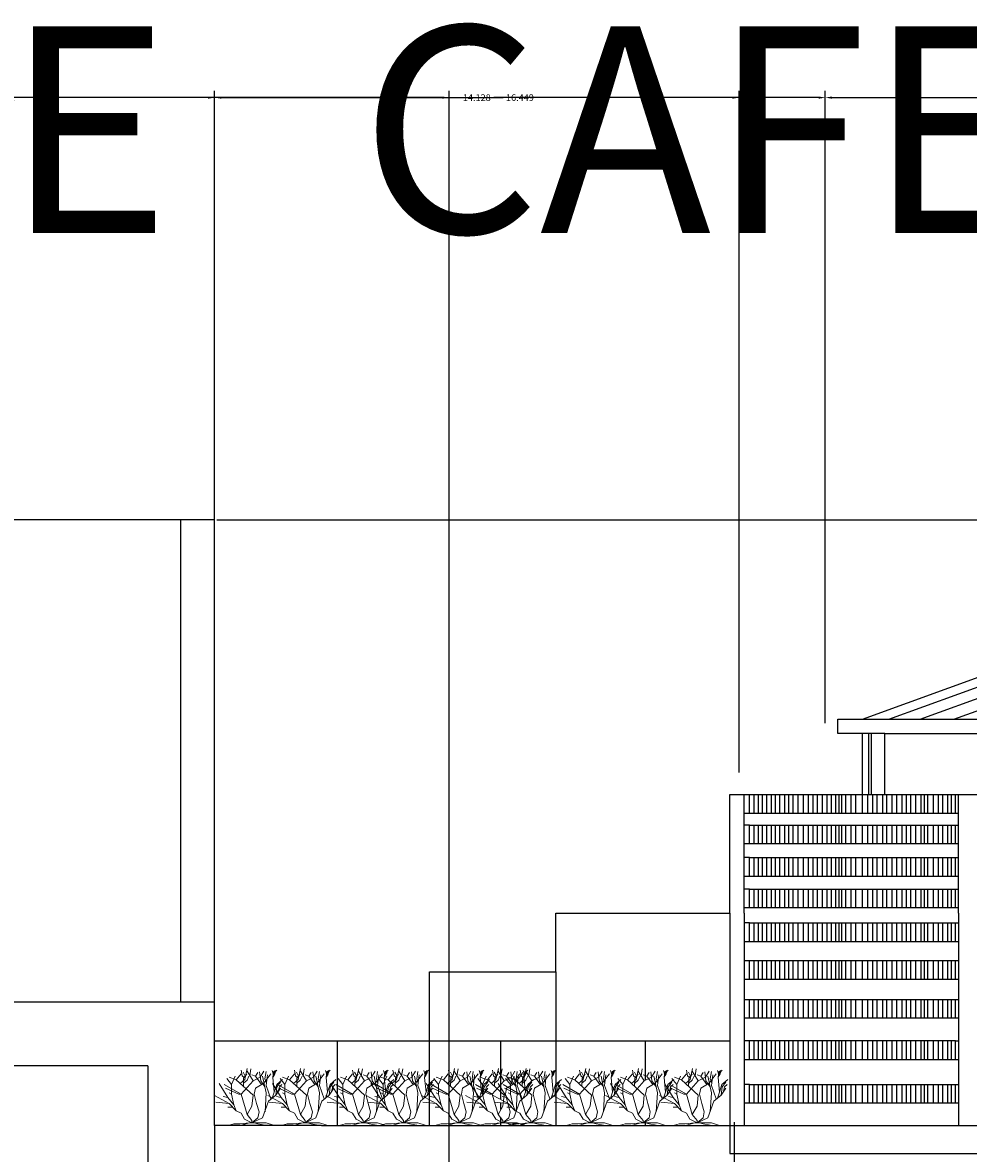
# Model space of a CAD drawing. Units: inches. Extents: x -117 to 121, y -77 to 40.
# Tile 30 of 45: x 9 to 34, y 10 to 40. Entities that reach past the tile are written whole.
import ezdxf

# ---------------------------------------------------------------- set-up
doc = ezdxf.new("R2010")
doc.units = ezdxf.units.IN
doc.header["$MEASUREMENT"] = 0
for name, color, linetype, lineweight in [('A-ANNO-DIMS', 2, 'Continuous', 18), ('A-ANNO-TEXT', 7, 'Continuous', 25), ('A-ELEV', 7, 'Continuous', 25), ('L-PLNT', 3, 'Continuous', 13)]:
    doc.layers.add(name, color=color, linetype=linetype, lineweight=lineweight)
doc.styles.get("Standard").update_dxf_attribs({"font": 'arial.ttf'})
doc.dimstyles.get("Standard").update_dxf_attribs({"dimtxt": 0.18, "dimasz": 0.18, "dimexe": 0.18, "dimexo": 0.0625, "dimgap": 0.09, "dimtad": 0, "dimtih": 1, "dimtoh": 1, "dimdec": 4, "dimzin": 0, "dimdsep": 46, "dimtxsty": 'Standard', "dimcen": 0.09, "dimadec": 0, "dimazin": 0, "dimtfac": 1, "dimtdec": 4, "dimtofl": 0, "dimtmove": 0, "dimatfit": 3, "dimfxl": 1, "dimtolj": 1, "dimtzin": 0, "dimarcsym": 0})

# ---------------------------------------------------------------- blocks, each defined once
blk = doc.blocks.new('*U3')
for p, q in [((-11.433, 18.289), (-10.457, 22.749)), ((-16.8, 16.32), (-18.72, 18.72)), ((-14.88, 18.24), (-17.76, 19.2)), ((-16.8, 16.32), (-15.36, 19.68)), ((-14.88, 18.24), (-12.96, 20.64)), ((-8.16, 12), (-14.88, 18.24)), ((-13.325, 16.724), (-11.433, 18.289)), ((-12.471, 19.775), (-12.898, 22.044)), ((-11.677, 19.071), (-12.471, 19.775)), ((-11.28, 19.619), (-12.104, 21.184)), ((-12.043, 15.628), (-11.921, 18.836)), ((-11.921, 18.836), (-10.64, 20.401)), ((-10.579, 18.054), (-9.846, 19.697)), ((-8.16, 17.76), (-10.56, 21.6)), ((-9.48, 19.775), (-8.992, 22.592)), ((-7.2, 19.68), (-8.64, 20.16)), ((-8.16, 17.76), (-5.28, 19.2)), ((-7.2, 19.68), (-6.24, 21.12)), ((-4.8, 16.32), (-7.2, 19.68)), ((-5.086, 17.741), (-5.513, 21.34)), ((-5.28, 19.2), (-3.84, 21.6)), ((-2.88, 12.96), (-4.32, 19.68)), ((-3.84, 16.8), (-0.96, 20.64)), ((-3.377, 18.602), (-2.888, 21.575)), ((-2.766, 16.802), (-3.377, 18.602)), ((-2.88, 15.84), (-2.4, 20.16)), ((-0.508, 21.888), (-0.081, 20.558)), ((-0.203, 19.149), (0.102, 21.34)), ((0.346, 13.203), (-0.203, 19.149)), ((-0.142, 19.384), (0.59, 20.401)), ((-0.02, 20.01), (0.896, 21.105)), ((0.041, 20.714), (1.384, 22.044)), ((0.102, 21.34), (0.835, 21.888)), ((1.323, 16.254), (3.642, 18.289)), ((-18.24, 11.04), (-21.755, 16.655)), ((-12.96, 12.48), (-19.68, 16.32)), ((-13.92, 12.48), (-19.2, 14.88)), ((-16.8, 12.48), (-16.8, 16.32)), ((-12.96, 12.48), (-8.16, 17.76)), ((-11.982, 16.802), (-10.579, 18.054)), ((-7.68, 12.48), (-7.2, 14.88)), ((-7.2, 14.88), (-3.84, 16.8)), ((-3.377, 15.315), (-5.086, 17.819)), ((-0.96, 10.56), (-2.88, 15.84)), ((0.346, 13.203), (1.323, 16.254)), ((0.96, 12), (1.44, 15.36)), ((0.96, 12), (2.88, 14.88)), ((1.44, 15.36), (2.88, 17.28)), ((1.92, 13.44), (2.4, 15.36)), ((2.4, 15.36), (3.36, 16.32)), ((-17.76, 8.64), (-23.663, 11.961)), ((-17.76, 8.64), (-23.128, 9.222)), ((-18.24, 11.04), (-20.16, 11.52)), ((-15.84, 8.16), (-18.24, 11.04)), ((-16.8, 12.48), (-17.76, 12.96)), ((-15.84, 8.16), (-16.8, 12.48)), ((-12.96, 12.48), (-13.92, 12.48)), ((-10.56, 4.32), (-12.96, 12.48)), ((-8.64, 7.68), (-8.16, 12)), ((-6.72, 8.64), (-7.68, 12.48)), ((-4.32, 2.88), (-1.92, 9.6)), ((-3.36, 5.28), (-2.88, 12.96)), ((-1.92, 9.6), (0.96, 12)), ((-0.48, 10.8), (0.346, 13.203)), ((-16.32, 7.2), (-18.24, 7.2)), ((-14.88, 5.76), (-17.76, 8.64)), ((-14.88, 5.76), (-15.84, 8.16)), ((-12.96, 4.8), (-14.88, 5.76)), ((-11.52, 2.4), (-12.96, 4.8)), ((-10.56, 4.32), (-8.64, 7.68)), ((-5.76, 5.28), (-6.72, 8.64)), ((-6.24, 2.88), (-5.76, 5.28)), ((-15.84, 0.48), (-17.76, 0)), ((-13.44, 0.48), (-15.84, 0.48)), ((-9.6, 0.96), (-13.44, 0.48)), ((-9.6, 0.96), (-12.96, 0)), ((-8.64, 0.96), (-11.52, 2.4)), ((-8.64, 1.92), (-10.56, 4.32)), ((-9.6, 0.96), (-7.68, 0.96)), ((-8.64, 0.96), (-4.32, 2.88)), ((-8.64, 0.96), (-6.24, 2.88)), ((-8.64, 0.96), (-8.64, 1.92)), ((-8.64, 0.96), (-2.88, 0.96)), ((-7.68, 0.96), (-6.24, 0.48)), ((-6.24, 0.48), (-3.36, 0)), ((-2.88, 0.96), (0, 0))]:
    blk.add_line(p, q)
blk = doc.blocks.new('*D10')
at = {"layer": 'A-ANNO-DIMS', "color": 0, "lineweight": -2, "transparency": 16777216}
for p, q in [((-2.6, 27.126), (-2.6, 38.61)), ((-2.42, 38.43), (5.304, 38.43)), ((13.798, 38.43), (6.075, 38.43)), ((13.978, 27.126), (13.978, 38.61))]:
    blk.add_line(p, q, dxfattribs=at)
at = {"layer": 'A-ANNO-DIMS', "color": 0, "transparency": 16777216}
for points in [[(-2.42, 38.46), (-2.42, 38.4), (-2.6, 38.43)], [(13.798, 38.46), (13.798, 38.4), (13.978, 38.43)]]:
    blk.add_solid(points, dxfattribs=at)
at = {"layer": 'Defpoints', "color": 0, "transparency": 16777216}
for p in [(13.978, 38.43), (-2.6, 27.063), (13.978, 27.063)]:
    blk.add_point(p, dxfattribs=at)
at = {"layer": 'A-ANNO-DIMS', "color": 0, "transparency": 16777216, "insert": (5.689, 38.43), "char_height": 0.18, "attachment_point": 5}
blk.add_mtext('\\A1;16.58', dxfattribs=at)
blk = doc.blocks.new('*D11')
at = {"layer": 'A-ANNO-DIMS', "color": 0, "lineweight": -2, "transparency": 16777216}
for p, q in [((30.428, 21.587), (30.428, 38.61)), ((30.608, 38.43), (50.217, 38.43)), ((70.62, 38.43), (51.011, 38.43)), ((70.8, 21.604), (70.8, 38.61))]:
    blk.add_line(p, q, dxfattribs=at)
at = {"layer": 'A-ANNO-DIMS', "color": 0, "transparency": 16777216}
for points in [[(30.608, 38.46), (30.608, 38.4), (30.428, 38.43)], [(70.62, 38.46), (70.62, 38.4), (70.8, 38.43)]]:
    blk.add_solid(points, dxfattribs=at)
at = {"layer": 'Defpoints', "color": 0, "transparency": 16777216}
for p in [(70.8, 38.43), (30.428, 21.525), (70.8, 21.541)]:
    blk.add_point(p, dxfattribs=at)
at = {"layer": 'A-ANNO-DIMS', "color": 0, "transparency": 16777216, "insert": (50.614, 38.43), "char_height": 0.18, "attachment_point": 5}
blk.add_mtext('\\A1;40.37', dxfattribs=at)
blk = doc.blocks.new('*D17')
at = {"layer": 'A-ANNO-DIMS', "color": 0, "lineweight": -2, "transparency": 16777216}
for p, q in [((14.041, 27.063), (120.84, 27.063)), ((120.66, 26.883), (120.66, 24.484)), ((120.66, 21.721), (120.66, 24.12)), ((70.862, 21.541), (120.84, 21.541))]:
    blk.add_line(p, q, dxfattribs=at)
at = {"layer": 'A-ANNO-DIMS', "color": 0, "transparency": 16777216}
for points in [[(120.63, 26.883), (120.69, 26.883), (120.66, 27.063)], [(120.63, 21.721), (120.69, 21.721), (120.66, 21.541)]]:
    blk.add_solid(points, dxfattribs=at)
at = {"layer": 'Defpoints', "color": 0, "transparency": 16777216}
for p in [(13.978, 27.063), (70.8, 21.541), (120.66, 21.541)]:
    blk.add_point(p, dxfattribs=at)
at = {"layer": 'A-ANNO-DIMS', "color": 0, "transparency": 16777216, "insert": (120.66, 24.302), "char_height": 0.18, "attachment_point": 5}
blk.add_mtext('\\A1;5.522', dxfattribs=at)
blk = doc.blocks.new('*D23')
at = {"layer": 'A-ANNO-DIMS', "color": 0, "lineweight": -2, "transparency": 16777216}
for p, q in [((13.978, 27.126), (13.978, 38.61)), ((14.158, 38.43), (21.748, 38.43)), ((30.248, 38.43), (22.658, 38.43)), ((30.428, 21.587), (30.428, 38.61))]:
    blk.add_line(p, q, dxfattribs=at)
at = {"layer": 'A-ANNO-DIMS', "color": 0, "transparency": 16777216}
for points in [[(14.158, 38.46), (14.158, 38.4), (13.978, 38.43)], [(30.248, 38.46), (30.248, 38.4), (30.428, 38.43)]]:
    blk.add_solid(points, dxfattribs=at)
at = {"layer": 'Defpoints', "color": 0, "transparency": 16777216}
for p in [(30.428, 38.43), (13.978, 27.063), (30.428, 21.525)]:
    blk.add_point(p, dxfattribs=at)
at = {"layer": 'A-ANNO-DIMS', "color": 0, "transparency": 16777216, "insert": (22.203, 38.43), "char_height": 0.18, "attachment_point": 5}
blk.add_mtext('\\A1;16.449', dxfattribs=at)
blk = doc.blocks.new('*D32')
at = {"layer": 'A-ANNO-DIMS', "color": 0, "lineweight": -2, "transparency": 16777216}
for p, q in [((-3.85, -45.55), (-3.85, 38.61)), ((-3.67, 38.43), (7.757, 38.43)), ((20.113, 38.43), (8.686, 38.43)), ((20.293, -45.55), (20.293, 38.61))]:
    blk.add_line(p, q, dxfattribs=at)
at = {"layer": 'A-ANNO-DIMS', "color": 0, "transparency": 16777216}
for points in [[(-3.67, 38.46), (-3.67, 38.4), (-3.85, 38.43)], [(20.113, 38.46), (20.113, 38.4), (20.293, 38.43)]]:
    blk.add_solid(points, dxfattribs=at)
at = {"layer": 'Defpoints', "color": 0, "transparency": 16777216}
for p in [(20.293, 38.43), (-3.85, -45.613), (20.293, -45.613)]:
    blk.add_point(p, dxfattribs=at)
at = {"layer": 'A-ANNO-DIMS', "color": 0, "transparency": 16777216, "insert": (8.222, 38.43), "char_height": 0.18, "attachment_point": 5}
blk.add_mtext('\\A1;24.142', dxfattribs=at)
blk = doc.blocks.new('*D51')
at = {"layer": 'A-ANNO-DIMS', "color": 0, "lineweight": -2, "transparency": 16777216}
for p, q in [((-22.563, 14.079), (-22.563, 38.61)), ((-22.383, 38.43), (-4.738, 38.43)), ((13.798, 38.43), (-3.846, 38.43)), ((13.978, 14.136), (13.978, 38.61))]:
    blk.add_line(p, q, dxfattribs=at)
at = {"layer": 'A-ANNO-DIMS', "color": 0, "transparency": 16777216}
for points in [[(-22.383, 38.46), (-22.383, 38.4), (-22.563, 38.43)], [(13.798, 38.46), (13.798, 38.4), (13.978, 38.43)]]:
    blk.add_solid(points, dxfattribs=at)
at = {"layer": 'Defpoints', "color": 0, "transparency": 16777216}
for p in [(13.978, 38.43), (-22.563, 14.016), (13.978, 14.074)]:
    blk.add_point(p, dxfattribs=at)
at = {"layer": 'A-ANNO-DIMS', "color": 0, "transparency": 16777216, "insert": (-4.292, 38.43), "char_height": 0.18, "attachment_point": 5}
blk.add_mtext('\\A1;36.541', dxfattribs=at)
blk = doc.blocks.new('*D52')
at = {"layer": 'A-ANNO-DIMS', "color": 0, "lineweight": -2, "transparency": 16777216}
for p, q in [((13.978, 14.136), (13.978, 38.61)), ((14.158, 38.43), (20.587, 38.43)), ((27.926, 38.43), (21.498, 38.43)), ((28.106, 20.256), (28.106, 38.61))]:
    blk.add_line(p, q, dxfattribs=at)
at = {"layer": 'A-ANNO-DIMS', "color": 0, "transparency": 16777216}
for points in [[(14.158, 38.46), (14.158, 38.4), (13.978, 38.43)], [(27.926, 38.46), (27.926, 38.4), (28.106, 38.43)]]:
    blk.add_solid(points, dxfattribs=at)
at = {"layer": 'Defpoints', "color": 0, "transparency": 16777216}
for p in [(28.106, 38.43), (28.106, 20.193), (13.978, 14.074)]:
    blk.add_point(p, dxfattribs=at)
at = {"layer": 'A-ANNO-DIMS', "color": 0, "transparency": 16777216, "insert": (21.042, 38.43), "char_height": 0.18, "attachment_point": 5}
blk.add_mtext('\\A1;14.128', dxfattribs=at)
blk = doc.blocks.new('*D53')
at = {"layer": 'A-ANNO-DIMS', "color": 0, "lineweight": -2, "transparency": 16777216}
for p, q in [((27.974, 10.841), (27.974, -77.193)), ((51.69, 10.9), (51.69, -77.193)), ((28.154, -77.013), (39.367, -77.013)), ((51.51, -77.013), (40.297, -77.013))]:
    blk.add_line(p, q, dxfattribs=at)
at = {"layer": 'A-ANNO-DIMS', "color": 0, "transparency": 16777216}
for points in [[(28.154, -76.983), (28.154, -77.043), (27.974, -77.013)], [(51.51, -76.983), (51.51, -77.043), (51.69, -77.013)]]:
    blk.add_solid(points, dxfattribs=at)
at = {"layer": 'Defpoints', "color": 0, "transparency": 16777216}
for p in [(51.69, 10.962), (27.974, 10.903), (51.69, -77.013)]:
    blk.add_point(p, dxfattribs=at)
at = {"layer": 'A-ANNO-DIMS', "color": 0, "transparency": 16777216, "insert": (39.832, -77.013), "char_height": 0.18, "attachment_point": 5}
blk.add_mtext('\\A1;23.716', dxfattribs=at)

msp = doc.modelspace()

# ---------------------------------------------------------------- linework, layer by layer
at = {"layer": 'A-ELEV'}
for p, q in [((13.9784, 27.0634), (-3.6347, 27.0634)), ((13.9784, 27.0634), (13.059, 27.0634)), ((13.059, 27.0634), (13.059, 14.0735)), ((13.9784, 14.0735), (13.9784, 27.0634)), ((31.4323, 21.689), (35.5367, 23.1855)), ((32.1361, 21.689), (35.6986, 22.9879)), ((32.9878, 21.689), (35.8604, 22.7364)), ((33.8934, 21.689), (36.0763, 22.4849)), ((30.7662, 21.3104), (30.7662, 21.689)), ((30.7662, 21.689), (70.6115, 21.689)), ((32.0351, 21.3104), (30.7662, 21.3104)), ((31.4323, 19.6653), (31.4323, 21.3104)), ((31.6045, 19.6653), (31.6045, 21.3104)), ((31.6691, 19.6653), (31.6691, 21.3104)), ((32.0351, 19.6653), (32.0351, 21.3104)), ((32.0351, 21.3104), (70.6115, 21.3104)), ((27.8529, 16.4655), (27.8529, 19.6653)), ((27.8529, 19.6653), (51.6089, 19.6653)), ((28.2472, 16.4655), (28.2472, 19.6653)), ((28.3894, 19.1644), (28.3894, 19.6653)), ((28.5115, 19.1644), (28.5115, 19.6653)), ((28.6258, 19.1644), (28.6258, 19.6653)), ((28.7402, 19.1644), (28.7402, 19.6653)), ((28.8546, 19.1644), (28.8546, 19.6653)), ((28.9767, 19.1644), (28.9767, 19.6653)), ((29.0834, 19.1644), (29.0834, 19.6653)), ((29.2054, 19.1644), (29.2054, 19.6653)), ((29.3351, 19.1644), (29.3351, 19.6653)), ((29.4495, 19.1644), (29.4495, 19.6653)), ((29.5639, 19.1644), (29.5639, 19.6653)), ((29.7011, 19.1644), (29.7011, 19.6653)), ((29.8384, 19.1644), (29.8384, 19.6653)), ((29.9757, 19.1644), (29.9757, 19.6653)), ((30.1053, 19.1644), (30.1053, 19.6653)), ((30.2197, 19.1644), (30.2197, 19.6653)), ((30.3494, 19.1644), (30.3494, 19.6653)), ((30.479, 19.1644), (30.479, 19.6653)), ((30.5934, 19.1644), (30.5934, 19.6653)), ((30.7154, 19.1644), (30.7154, 19.6653)), ((30.8032, 19.1644), (30.8032, 19.6562)), ((30.8756, 19.1644), (30.8756, 19.6653)), ((30.9823, 19.1644), (30.9823, 19.6653)), ((31.1272, 19.1644), (31.1272, 19.6653)), ((31.2493, 19.1644), (31.2493, 19.6653)), ((31.4323, 19.1644), (31.4323, 19.6653)), ((31.5696, 19.1644), (31.5696, 19.6653)), ((31.7068, 19.1644), (31.7068, 19.6653)), ((31.8288, 19.1644), (31.8288, 19.6653)), ((31.9737, 19.1644), (31.9737, 19.6653)), ((32.0881, 19.1644), (32.0881, 19.6653)), ((32.233, 19.1644), (32.233, 19.6653)), ((32.3551, 19.1644), (32.3551, 19.6653)), ((32.5, 19.1644), (32.5, 19.6653)), ((32.6143, 19.1644), (32.6143, 19.6653)), ((32.7364, 19.1644), (32.7364, 19.6653)), ((32.866, 19.1644), (32.866, 19.6653)), ((33.0109, 19.1644), (33.0109, 19.6653)), ((33.1024, 19.1644), (33.1024, 19.6653)), ((33.1939, 19.1644), (33.1939, 19.6653)), ((33.3465, 19.1644), (33.3465, 19.6653)), ((33.4761, 19.1644), (33.4761, 19.6653)), ((33.5981, 19.1644), (33.5981, 19.6653)), ((33.7278, 19.1644), (33.7278, 19.6653)), ((33.8269, 19.1644), (33.8269, 19.6653)), ((33.9337, 19.1644), (33.9337, 19.6653)), ((34.0136, 16.4655), (34.0136, 19.6653)), ((28.2472, 19.1644), (34.0136, 19.1644)), ((28.3894, 18.8424), (28.2472, 18.8424)), ((28.3894, 18.3415), (28.3894, 18.8424)), ((28.3894, 18.8424), (34.0136, 18.8424)), ((28.5115, 18.3415), (28.5115, 18.8424)), ((28.6258, 18.3415), (28.6258, 18.8424)), ((28.7402, 18.3415), (28.7402, 18.8424)), ((28.8546, 18.3415), (28.8546, 18.8424)), ((28.9767, 18.3415), (28.9767, 18.8424)), ((29.0834, 18.3415), (29.0834, 18.8424)), ((29.2054, 18.3415), (29.2054, 18.8424)), ((29.3351, 18.3415), (29.3351, 18.8424)), ((29.4495, 18.3415), (29.4495, 18.8424)), ((29.5639, 18.3415), (29.5639, 18.8424)), ((29.7011, 18.3415), (29.7011, 18.8424)), ((29.8384, 18.3415), (29.8384, 18.8424)), ((29.9757, 18.3415), (29.9757, 18.8424)), ((30.1053, 18.3415), (30.1053, 18.8424)), ((30.2197, 18.3415), (30.2197, 18.8424)), ((30.3494, 18.3415), (30.3494, 18.8424)), ((30.479, 18.3415), (30.479, 18.8424)), ((30.5934, 18.3415), (30.5934, 18.8424)), ((30.7154, 18.3415), (30.7154, 18.8424)), ((30.8032, 18.3415), (30.8032, 18.8333)), ((30.8756, 18.3415), (30.8756, 18.8424)), ((30.9823, 18.3415), (30.9823, 18.8424)), ((31.1272, 18.3415), (31.1272, 18.8424)), ((31.2493, 18.3415), (31.2493, 18.8424)), ((31.4323, 18.3415), (31.4323, 18.8424)), ((31.5696, 18.3415), (31.5696, 18.8424)), ((31.7068, 18.3415), (31.7068, 18.8424)), ((31.8288, 18.3415), (31.8288, 18.8424)), ((31.9737, 18.3415), (31.9737, 18.8424)), ((32.0881, 18.3415), (32.0881, 18.8424)), ((32.233, 18.3415), (32.233, 18.8424)), ((32.3551, 18.3415), (32.3551, 18.8424)), ((32.5, 18.3415), (32.5, 18.8424)), ((32.6143, 18.3415), (32.6143, 18.8424)), ((32.7364, 18.3415), (32.7364, 18.8424)), ((32.866, 18.3415), (32.866, 18.8424)), ((33.0109, 18.3415), (33.0109, 18.8424)), ((33.1024, 18.3415), (33.1024, 18.8424)), ((33.1939, 18.3415), (33.1939, 18.8424)), ((33.3465, 18.3415), (33.3465, 18.8424)), ((33.4761, 18.3415), (33.4761, 18.8424)), ((33.5981, 18.3415), (33.5981, 18.8424)), ((33.7278, 18.3415), (33.7278, 18.8424)), ((33.8269, 18.3415), (33.8269, 18.8424)), ((33.9337, 18.3415), (33.9337, 18.8424)), ((28.2472, 18.3415), (34.0136, 18.3415)), ((28.3894, 17.9696), (28.2472, 17.9696)), ((28.3894, 17.4687), (28.3894, 17.9696)), ((28.3894, 17.9696), (34.0136, 17.9696)), ((28.5115, 17.4687), (28.5115, 17.9696)), ((28.6258, 17.4687), (28.6258, 17.9696)), ((28.7402, 17.4687), (28.7402, 17.9696)), ((28.8546, 17.4687), (28.8546, 17.9696)), ((28.9767, 17.4687), (28.9767, 17.9696)), ((29.0834, 17.4687), (29.0834, 17.9696)), ((29.2054, 17.4687), (29.2054, 17.9696)), ((29.3351, 17.4687), (29.3351, 17.9696)), ((29.4495, 17.4687), (29.4495, 17.9696)), ((29.5639, 17.4687), (29.5639, 17.9696)), ((29.7011, 17.4687), (29.7011, 17.9696)), ((29.8384, 17.4687), (29.8384, 17.9696)), ((29.9757, 17.4687), (29.9757, 17.9696)), ((30.1053, 17.4687), (30.1053, 17.9696)), ((30.2197, 17.4687), (30.2197, 17.9696)), ((30.3494, 17.4687), (30.3494, 17.9696)), ((30.479, 17.4687), (30.479, 17.9696)), ((30.5934, 17.4687), (30.5934, 17.9696)), ((30.7154, 17.4687), (30.7154, 17.9696)), ((30.8756, 17.4687), (30.8756, 17.9696)), ((30.9823, 17.4687), (30.9823, 17.9696)), ((31.1272, 17.4687), (31.1272, 17.9696)), ((31.2493, 17.4687), (31.2493, 17.9696)), ((31.4323, 17.4687), (31.4323, 17.9696)), ((31.5696, 17.4687), (31.5696, 17.9696)), ((31.7068, 17.4687), (31.7068, 17.9696)), ((31.8288, 17.4687), (31.8288, 17.9696)), ((31.9737, 17.4687), (31.9737, 17.9696)), ((32.0881, 17.4687), (32.0881, 17.9696)), ((32.233, 17.4687), (32.233, 17.9696)), ((32.3551, 17.4687), (32.3551, 17.9696)), ((32.5, 17.4687), (32.5, 17.9696)), ((32.6143, 17.4687), (32.6143, 17.9696)), ((32.7364, 17.4687), (32.7364, 17.9696)), ((32.866, 17.4687), (32.866, 17.9696)), ((33.0109, 17.4687), (33.0109, 17.9696)), ((33.1024, 17.4687), (33.1024, 17.9696)), ((33.1939, 17.4687), (33.1939, 17.9696)), ((33.3465, 17.4687), (33.3465, 17.9696)), ((33.4761, 17.4687), (33.4761, 17.9696)), ((33.5981, 17.4687), (33.5981, 17.9696)), ((33.7278, 17.4687), (33.7278, 17.9696)), ((33.8269, 17.4687), (33.8269, 17.9696)), ((33.9337, 17.4687), (33.9337, 17.9696)), ((30.8032, 17.4687), (30.8032, 17.9605)), ((28.2472, 17.4687), (34.0136, 17.4687)), ((28.3894, 17.1187), (28.2472, 17.1187)), ((28.3894, 16.6179), (28.3894, 17.1187)), ((28.3894, 17.1187), (34.0136, 17.1187)), ((28.5115, 16.6179), (28.5115, 17.1187)), ((28.6258, 16.6179), (28.6258, 17.1187)), ((28.7402, 16.6179), (28.7402, 17.1187)), ((28.8546, 16.6179), (28.8546, 17.1187)), ((28.9767, 16.6179), (28.9767, 17.1187)), ((29.0834, 16.6179), (29.0834, 17.1187)), ((29.2054, 16.6179), (29.2054, 17.1187)), ((29.3351, 16.6179), (29.3351, 17.1187)), ((29.4495, 16.6179), (29.4495, 17.1187)), ((29.5639, 16.6179), (29.5639, 17.1187)), ((29.7011, 16.6179), (29.7011, 17.1187)), ((29.8384, 16.6179), (29.8384, 17.1187)), ((29.9757, 16.6179), (29.9757, 17.1187)), ((30.1053, 16.6179), (30.1053, 17.1187)), ((30.2197, 16.6179), (30.2197, 17.1187)), ((30.3494, 16.6179), (30.3494, 17.1187)), ((30.479, 16.6179), (30.479, 17.1187)), ((30.5934, 16.6179), (30.5934, 17.1187)), ((30.7154, 16.6179), (30.7154, 17.1187)), ((30.8032, 16.6179), (30.8032, 17.1097)), ((30.8756, 16.6179), (30.8756, 17.1187)), ((30.9823, 16.6179), (30.9823, 17.1187)), ((31.1272, 16.6179), (31.1272, 17.1187)), ((31.2493, 16.6179), (31.2493, 17.1187)), ((31.4323, 16.6179), (31.4323, 17.1187)), ((31.5696, 16.6179), (31.5696, 17.1187)), ((31.7068, 16.6179), (31.7068, 17.1187)), ((31.8288, 16.6179), (31.8288, 17.1187)), ((31.9737, 16.6179), (31.9737, 17.1187)), ((32.0881, 16.6179), (32.0881, 17.1187)), ((32.233, 16.6179), (32.233, 17.1187)), ((32.3551, 16.6179), (32.3551, 17.1187)), ((32.5, 16.6179), (32.5, 17.1187)), ((32.6143, 16.6179), (32.6143, 17.1187)), ((32.7364, 16.6179), (32.7364, 17.1187)), ((32.866, 16.6179), (32.866, 17.1187)), ((33.0109, 16.6179), (33.0109, 17.1187)), ((33.1024, 16.6179), (33.1024, 17.1187)), ((33.1939, 16.6179), (33.1939, 17.1187)), ((33.3465, 16.6179), (33.3465, 17.1187)), ((33.4761, 16.6179), (33.4761, 17.1187)), ((33.5981, 16.6179), (33.5981, 17.1187)), ((33.7278, 16.6179), (33.7278, 17.1187)), ((33.8269, 16.6179), (33.8269, 17.1187)), ((33.9337, 16.6179), (33.9337, 17.1187)), ((23.1707, 14.8902), (23.1707, 16.4655)), ((23.1707, 16.4655), (27.8529, 16.4655)), ((27.8529, 16.4655), (27.8529, 10.755)), ((28.2472, 16.6179), (34.0136, 16.6179)), ((28.2472, 16.4655), (28.2472, 10.755)), ((34.0136, 16.4655), (34.0136, 10.755)), ((28.3894, 16.2085), (28.2472, 16.2085)), ((28.3894, 15.7077), (28.3894, 16.2085)), ((28.3894, 16.2085), (34.0136, 16.2085)), ((28.5115, 15.7077), (28.5115, 16.2085)), ((28.6258, 15.7077), (28.6258, 16.2085)), ((28.7402, 15.7077), (28.7402, 16.2085)), ((28.8546, 15.7077), (28.8546, 16.2085)), ((28.9767, 15.7077), (28.9767, 16.2085)), ((29.0834, 15.7077), (29.0834, 16.2085)), ((29.2054, 15.7077), (29.2054, 16.2085)), ((29.3351, 15.7077), (29.3351, 16.2085)), ((29.4495, 15.7077), (29.4495, 16.2085)), ((29.5639, 15.7077), (29.5639, 16.2085)), ((29.7011, 15.7077), (29.7011, 16.2085)), ((29.8384, 15.7077), (29.8384, 16.2085)), ((29.9757, 15.7077), (29.9757, 16.2085)), ((30.1053, 15.7077), (30.1053, 16.2085)), ((30.2197, 15.7077), (30.2197, 16.2085)), ((30.3494, 15.7077), (30.3494, 16.2085)), ((30.479, 15.7077), (30.479, 16.2085)), ((30.5934, 15.7077), (30.5934, 16.2085)), ((30.7154, 15.7077), (30.7154, 16.2085)), ((30.8032, 15.7077), (30.8032, 16.1995)), ((30.8756, 15.7077), (30.8756, 16.2085)), ((30.9823, 15.7077), (30.9823, 16.2085)), ((31.1272, 15.7077), (31.1272, 16.2085)), ((31.2493, 15.7077), (31.2493, 16.2085)), ((31.4323, 15.7077), (31.4323, 16.2085)), ((31.5696, 15.7077), (31.5696, 16.2085)), ((31.7068, 15.7077), (31.7068, 16.2085)), ((31.8288, 15.7077), (31.8288, 16.2085)), ((31.9737, 15.7077), (31.9737, 16.2085)), ((32.0881, 15.7077), (32.0881, 16.2085)), ((32.233, 15.7077), (32.233, 16.2085)), ((32.3551, 15.7077), (32.3551, 16.2085)), ((32.5, 15.7077), (32.5, 16.2085)), ((32.6143, 15.7077), (32.6143, 16.2085)), ((32.7364, 15.7077), (32.7364, 16.2085)), ((32.866, 15.7077), (32.866, 16.2085)), ((33.0109, 15.7077), (33.0109, 16.2085)), ((33.1024, 15.7077), (33.1024, 16.2085)), ((33.1939, 15.7077), (33.1939, 16.2085)), ((33.3465, 15.7077), (33.3465, 16.2085)), ((33.4761, 15.7077), (33.4761, 16.2085)), ((33.5981, 15.7077), (33.5981, 16.2085)), ((33.7278, 15.7077), (33.7278, 16.2085)), ((33.8269, 15.7077), (33.8269, 16.2085)), ((33.9337, 15.7077), (33.9337, 16.2085)), ((28.2472, 15.7077), (34.0136, 15.7077)), ((28.2472, 15.1944), (34.0136, 15.1944)), ((28.3894, 14.6936), (28.3894, 15.1944)), ((28.5115, 14.6936), (28.5115, 15.1944)), ((28.6258, 14.6936), (28.6258, 15.1944)), ((28.7402, 14.6936), (28.7402, 15.1944)), ((28.8546, 14.6936), (28.8546, 15.1944)), ((28.9767, 14.6936), (28.9767, 15.1944)), ((29.0834, 14.6936), (29.0834, 15.1944)), ((29.2054, 14.6936), (29.2054, 15.1944)), ((29.3351, 14.6936), (29.3351, 15.1944)), ((29.4495, 14.6936), (29.4495, 15.1944)), ((29.5639, 14.6936), (29.5639, 15.1944)), ((29.7011, 14.6936), (29.7011, 15.1944)), ((29.8384, 14.6936), (29.8384, 15.1944)), ((29.9757, 14.6936), (29.9757, 15.1944)), ((30.1053, 14.6936), (30.1053, 15.1944)), ((30.2197, 14.6936), (30.2197, 15.1944)), ((30.3494, 14.6936), (30.3494, 15.1944)), ((30.479, 14.6936), (30.479, 15.1944)), ((30.5934, 14.6936), (30.5934, 15.1944)), ((30.7154, 14.6936), (30.7154, 15.1944)), ((30.8032, 14.6936), (30.8032, 15.1854)), ((30.8756, 14.6936), (30.8756, 15.1944)), ((30.9823, 14.6936), (30.9823, 15.1944)), ((31.1272, 14.6936), (31.1272, 15.1944)), ((31.2493, 14.6936), (31.2493, 15.1944)), ((31.4323, 14.6936), (31.4323, 15.1944)), ((31.5696, 14.6936), (31.5696, 15.1944)), ((31.7068, 14.6936), (31.7068, 15.1944)), ((31.8288, 14.6936), (31.8288, 15.1944)), ((31.9737, 14.6936), (31.9737, 15.1944)), ((32.0881, 14.6936), (32.0881, 15.1944)), ((32.233, 14.6936), (32.233, 15.1944)), ((32.3551, 14.6936), (32.3551, 15.1944)), ((32.5, 14.6936), (32.5, 15.1944)), ((32.6143, 14.6936), (32.6143, 15.1944)), ((32.7364, 14.6936), (32.7364, 15.1944)), ((32.866, 14.6936), (32.866, 15.1944)), ((33.0109, 14.6936), (33.0109, 15.1944)), ((33.1024, 14.6936), (33.1024, 15.1944)), ((33.1939, 14.6936), (33.1939, 15.1944)), ((33.3465, 14.6936), (33.3465, 15.1944)), ((33.4761, 14.6936), (33.4761, 15.1944)), ((33.5981, 14.6936), (33.5981, 15.1944)), ((33.7278, 14.6936), (33.7278, 15.1944)), ((33.8269, 14.6936), (33.8269, 15.1944)), ((33.9337, 14.6936), (33.9337, 15.1944)), ((19.7699, 10.755), (19.7699, 14.8902)), ((19.7699, 14.8902), (23.1707, 14.8902)), ((23.1707, 14.8902), (23.1707, 10.755)), ((28.2472, 14.6936), (34.0136, 14.6936)), ((13.9784, 14.0735), (-11.738, 14.0735)), ((13.9784, 13.0312), (13.9784, 14.0735)), ((28.2472, 14.1471), (34.0136, 14.1471)), ((28.3894, 13.6462), (28.3894, 14.1471)), ((28.5115, 13.6462), (28.5115, 14.1471)), ((28.6258, 13.6462), (28.6258, 14.1471)), ((28.7402, 13.6462), (28.7402, 14.1471)), ((28.8546, 13.6462), (28.8546, 14.1471)), ((28.9767, 13.6462), (28.9767, 14.1471)), ((29.0834, 13.6462), (29.0834, 14.1471)), ((29.2054, 13.6462), (29.2054, 14.1471)), ((29.3351, 13.6462), (29.3351, 14.1471)), ((29.4495, 13.6462), (29.4495, 14.1471)), ((29.5639, 13.6462), (29.5639, 14.1471)), ((29.7011, 13.6462), (29.7011, 14.1471)), ((29.8384, 13.6462), (29.8384, 14.1471)), ((29.9757, 13.6462), (29.9757, 14.1471)), ((30.1053, 13.6462), (30.1053, 14.1471)), ((30.2197, 13.6462), (30.2197, 14.1471)), ((30.3494, 13.6462), (30.3494, 14.1471)), ((30.479, 13.6462), (30.479, 14.1471)), ((30.5934, 13.6462), (30.5934, 14.1471)), ((30.7154, 13.6462), (30.7154, 14.1471)), ((30.8032, 13.6462), (30.8032, 14.138)), ((30.8756, 13.6462), (30.8756, 14.1471)), ((30.9823, 13.6462), (30.9823, 14.1471)), ((31.1272, 13.6462), (31.1272, 14.1471)), ((31.2493, 13.6462), (31.2493, 14.1471)), ((31.4323, 13.6462), (31.4323, 14.1471)), ((31.5696, 13.6462), (31.5696, 14.1471)), ((31.7068, 13.6462), (31.7068, 14.1471)), ((31.8288, 13.6462), (31.8288, 14.1471)), ((31.9737, 13.6462), (31.9737, 14.1471)), ((32.0881, 13.6462), (32.0881, 14.1471)), ((32.233, 13.6462), (32.233, 14.1471)), ((32.3551, 13.6462), (32.3551, 14.1471)), ((32.5, 13.6462), (32.5, 14.1471)), ((32.6143, 13.6462), (32.6143, 14.1471)), ((32.7364, 13.6462), (32.7364, 14.1471)), ((32.866, 13.6462), (32.866, 14.1471)), ((33.0109, 13.6462), (33.0109, 14.1471)), ((33.1024, 13.6462), (33.1024, 14.1471)), ((33.1939, 13.6462), (33.1939, 14.1471)), ((33.3465, 13.6462), (33.3465, 14.1471)), ((33.4761, 13.6462), (33.4761, 14.1471)), ((33.5981, 13.6462), (33.5981, 14.1471)), ((33.7278, 13.6462), (33.7278, 14.1471)), ((33.8269, 13.6462), (33.8269, 14.1471)), ((33.9337, 13.6462), (33.9337, 14.1471)), ((28.2472, 13.6462), (34.0136, 13.6462)), ((13.9784, 13.0312), (27.8529, 13.0312)), ((13.9784, 10.755), (13.9784, 13.0312)), ((17.2893, 10.755), (17.2893, 13.0312)), ((21.6916, 11.4473), (21.6916, 13.0312)), ((25.5846, 11.9682), (25.5846, 13.0312)), ((33.9337, 13.0312), (28.2472, 13.0312)), ((28.3894, 12.5304), (28.3894, 13.0312)), ((28.5115, 12.5304), (28.5115, 13.0312)), ((28.6258, 12.5304), (28.6258, 13.0312)), ((28.7402, 12.5304), (28.7402, 13.0312)), ((28.8546, 12.5304), (28.8546, 13.0312)), ((28.9767, 12.5304), (28.9767, 13.0312)), ((29.0834, 12.5304), (29.0834, 13.0312)), ((29.2054, 12.5304), (29.2054, 13.0312)), ((29.3351, 12.5304), (29.3351, 13.0312)), ((29.4495, 12.5304), (29.4495, 13.0312)), ((29.5639, 12.5304), (29.5639, 13.0312)), ((29.7011, 12.5304), (29.7011, 13.0312)), ((29.8384, 12.5304), (29.8384, 13.0312)), ((29.9757, 12.5304), (29.9757, 13.0312)), ((30.1053, 12.5304), (30.1053, 13.0312)), ((30.2197, 12.5304), (30.2197, 13.0312)), ((30.3494, 12.5304), (30.3494, 13.0312)), ((30.479, 12.5304), (30.479, 13.0312)), ((30.5934, 12.5304), (30.5934, 13.0312)), ((30.7154, 12.5304), (30.7154, 13.0312)), ((30.8032, 12.5304), (30.8032, 13.0221)), ((30.8756, 12.5304), (30.8756, 13.0312)), ((30.9823, 12.5304), (30.9823, 13.0312)), ((31.1272, 12.5304), (31.1272, 13.0312)), ((31.2493, 12.5304), (31.2493, 13.0312)), ((31.4323, 12.5304), (31.4323, 13.0312)), ((31.5696, 12.5304), (31.5696, 13.0312)), ((31.7068, 12.5304), (31.7068, 13.0312)), ((31.8288, 12.5304), (31.8288, 13.0312)), ((31.9737, 12.5304), (31.9737, 13.0312)), ((32.0881, 12.5304), (32.0881, 13.0312)), ((32.233, 12.5304), (32.233, 13.0312)), ((32.3551, 12.5304), (32.3551, 13.0312)), ((32.5, 12.5304), (32.5, 13.0312)), ((32.6143, 12.5304), (32.6143, 13.0312)), ((32.7364, 12.5304), (32.7364, 13.0312)), ((32.866, 12.5304), (32.866, 13.0312)), ((33.0109, 12.5304), (33.0109, 13.0312)), ((33.1024, 12.5304), (33.1024, 13.0312)), ((33.1939, 12.5304), (33.1939, 13.0312)), ((33.3465, 12.5304), (33.3465, 13.0312)), ((33.4761, 12.5304), (33.4761, 13.0312)), ((33.5981, 12.5304), (33.5981, 13.0312)), ((33.7278, 12.5304), (33.7278, 13.0312)), ((33.8269, 12.5304), (33.8269, 13.0312)), ((33.9337, 12.5304), (33.9337, 13.0312)), ((33.9337, 13.0312), (34.0136, 13.0312)), ((28.2472, 12.5304), (34.0136, 12.5304)), ((12.1837, 12.3611), (-10.1416, 12.3611)), ((12.1837, 12.3611), (12.1837, 5.6232)), ((28.3894, 11.8591), (28.2472, 11.8591)), ((28.3894, 11.3583), (28.3894, 11.8591)), ((28.3894, 11.8591), (34.0136, 11.8591)), ((28.5115, 11.3583), (28.5115, 11.8591)), ((28.6258, 11.3583), (28.6258, 11.8591)), ((28.7402, 11.3583), (28.7402, 11.8591)), ((28.8546, 11.3583), (28.8546, 11.8591)), ((28.9767, 11.3583), (28.9767, 11.8591)), ((29.0834, 11.3583), (29.0834, 11.8591)), ((29.2054, 11.3583), (29.2054, 11.8591)), ((29.3351, 11.3583), (29.3351, 11.8591)), ((29.4495, 11.3583), (29.4495, 11.8591)), ((29.5639, 11.3583), (29.5639, 11.8591)), ((29.7011, 11.3583), (29.7011, 11.8591)), ((29.8384, 11.3583), (29.8384, 11.8591)), ((29.9757, 11.3583), (29.9757, 11.8591)), ((30.1053, 11.3583), (30.1053, 11.8591)), ((30.2197, 11.3583), (30.2197, 11.8591)), ((30.3494, 11.3583), (30.3494, 11.8591)), ((30.479, 11.3583), (30.479, 11.8591)), ((30.5934, 11.3583), (30.5934, 11.8591)), ((30.7154, 11.3583), (30.7154, 11.8591)), ((30.8032, 11.3583), (30.8032, 11.8501)), ((30.8756, 11.3583), (30.8756, 11.8591)), ((30.9823, 11.3583), (30.9823, 11.8591)), ((31.1272, 11.3583), (31.1272, 11.8591)), ((31.2493, 11.3583), (31.2493, 11.8591)), ((31.4323, 11.3583), (31.4323, 11.8591)), ((31.5696, 11.3583), (31.5696, 11.8591)), ((31.7068, 11.3583), (31.7068, 11.8591)), ((31.8288, 11.3583), (31.8288, 11.8591)), ((31.9737, 11.3583), (31.9737, 11.8591)), ((32.0881, 11.3583), (32.0881, 11.8591)), ((32.233, 11.3583), (32.233, 11.8591)), ((32.3551, 11.3583), (32.3551, 11.8591)), ((32.5, 11.3583), (32.5, 11.8591)), ((32.6143, 11.3583), (32.6143, 11.8591)), ((32.7364, 11.3583), (32.7364, 11.8591)), ((32.866, 11.3583), (32.866, 11.8591)), ((33.0109, 11.3583), (33.0109, 11.8591)), ((33.1024, 11.3583), (33.1024, 11.8591)), ((33.1939, 11.3583), (33.1939, 11.8591)), ((33.3465, 11.3583), (33.3465, 11.8591)), ((33.4761, 11.3583), (33.4761, 11.8591)), ((33.5981, 11.3583), (33.5981, 11.8591)), ((33.7278, 11.3583), (33.7278, 11.8591)), ((33.8269, 11.3583), (33.8269, 11.8591)), ((33.9337, 11.3583), (33.9337, 11.8591)), ((21.6916, 11.1805), (21.6916, 11.3606)), ((28.2472, 11.3583), (34.0136, 11.3583)), ((16.862, 10.755), (13.9784, 10.755)), ((13.9784, 10.755), (13.9784, 5.623)), ((16.862, 10.755), (51.6089, 10.755)), ((21.6916, 10.755), (21.6916, 10.9564)), ((25.5846, 10.755), (25.5846, 10.8751)), ((27.8529, 10.755), (27.8529, 9.9998)), ((27.8529, 9.9998), (57.6104, 9.9998))]:
    msp.add_line(p, q, dxfattribs=at)

# ---------------------------------------------------------------- block references
at = {"layer": 'L-PLNT', "xscale": 0.0671647796176818, "yscale": 0.0671647796176818, "zscale": 0.0671647796176818}
for p in [(15.5621, 10.7596), (16.9984, 10.7596), (18.5637, 10.7596), (19.6502, 10.7596), (21.1417, 10.7596), (22.3262, 10.7596), (23.0753, 10.7596), (24.6774, 10.7596), (26.1012, 10.7596), (27.5559, 10.7596)]:
    msp.add_blockref('*U3', p, dxfattribs=at)

# ---------------------------------------------------------------- texts
at = {"layer": 'A-ANNO-TEXT'}
msp.add_text('CONCEPTUAL    GOOD   VIBE   CAFE   DESIGN', height=5.56486, dxfattribs=at).set_placement((-85.726, 34.7863))

# ---------------------------------------------------------------- dimensions: what is measured, and where the dimension line sits
at = {"layer": 'A-ANNO-DIMS'}
for base, p1, p2, override, picture, middle in [((13.9784, 38.4297), (-22.5628, 14.0161), (13.9784, 14.0735), {"dimdec": 3, "dimlfac": 1, "dimrnd": 0, "dimzin": 0, "dimdsep": 46, "dimlunit": 2}, '*D51', (-4.2922, 38.4297)), ((20.2929, 38.4297), (-3.8495, -45.6125), (20.2929, -45.6125), {"dimdec": 3, "dimlfac": 1, "dimrnd": 0, "dimzin": 0, "dimdsep": 46, "dimlunit": 2}, '*D32', (8.2217, 38.4297)), ((13.9784, 38.4297), (-2.6001, 27.0634), (13.9784, 27.0634), {"dimdec": 2, "dimlfac": 1, "dimrnd": 0, "dimzin": 0, "dimdsep": 46, "dimlunit": 2}, '*D10', (5.6892, 38.4297)), ((30.4277, 38.4297), (13.9784, 27.0634), (30.4277, 21.5247), {"dimdec": 3, "dimlfac": 1, "dimrnd": 0, "dimzin": 0, "dimdsep": 46, "dimlunit": 2}, '*D23', (22.2031, 38.4297)), ((28.1064, 38.4297), (13.9784, 14.0735), (28.1064, 20.1933), {"dimdec": 3, "dimlfac": 1, "dimrnd": 0, "dimzin": 0, "dimdsep": 46, "dimlunit": 2}, '*D52', (21.0424, 38.4297)), ((70.8, 38.4297), (30.4277, 21.5247), (70.8, 21.5414), {"dimdec": 2, "dimlfac": 1, "dimrnd": 0, "dimzin": 0, "dimdsep": 46, "dimlunit": 2}, '*D11', (50.6138, 38.4297)), ((51.6901, -77.0135), (27.9744, 10.9032), (51.6901, 10.9623), {"dimdec": 3, "dimlfac": 1, "dimrnd": 0, "dimzin": 0, "dimdsep": 46, "dimlunit": 2}, '*D53', (39.8322, -77.0135))]:
    dim = msp.add_linear_dim(base=base, p1=p1, p2=p2, dimstyle='Standard', override=override, dxfattribs=at)
    dim.commit()
    dim.dimension.update_dxf_attribs({"geometry": picture, "text_midpoint": middle})
dim = msp.add_linear_dim(base=(120.6602, 21.5414), p1=(13.9784, 27.0634), p2=(70.8, 21.5414), angle=90, dimstyle='Standard', override={"dimdec": 3, "dimlfac": 1, "dimrnd": 0, "dimzin": 0, "dimdsep": 46, "dimlunit": 2}, dxfattribs=at)
dim.commit()
dim.dimension.update_dxf_attribs({"geometry": '*D17', "text_midpoint": (120.6602, 24.3024)})

doc.saveas('drawing.dxf')
